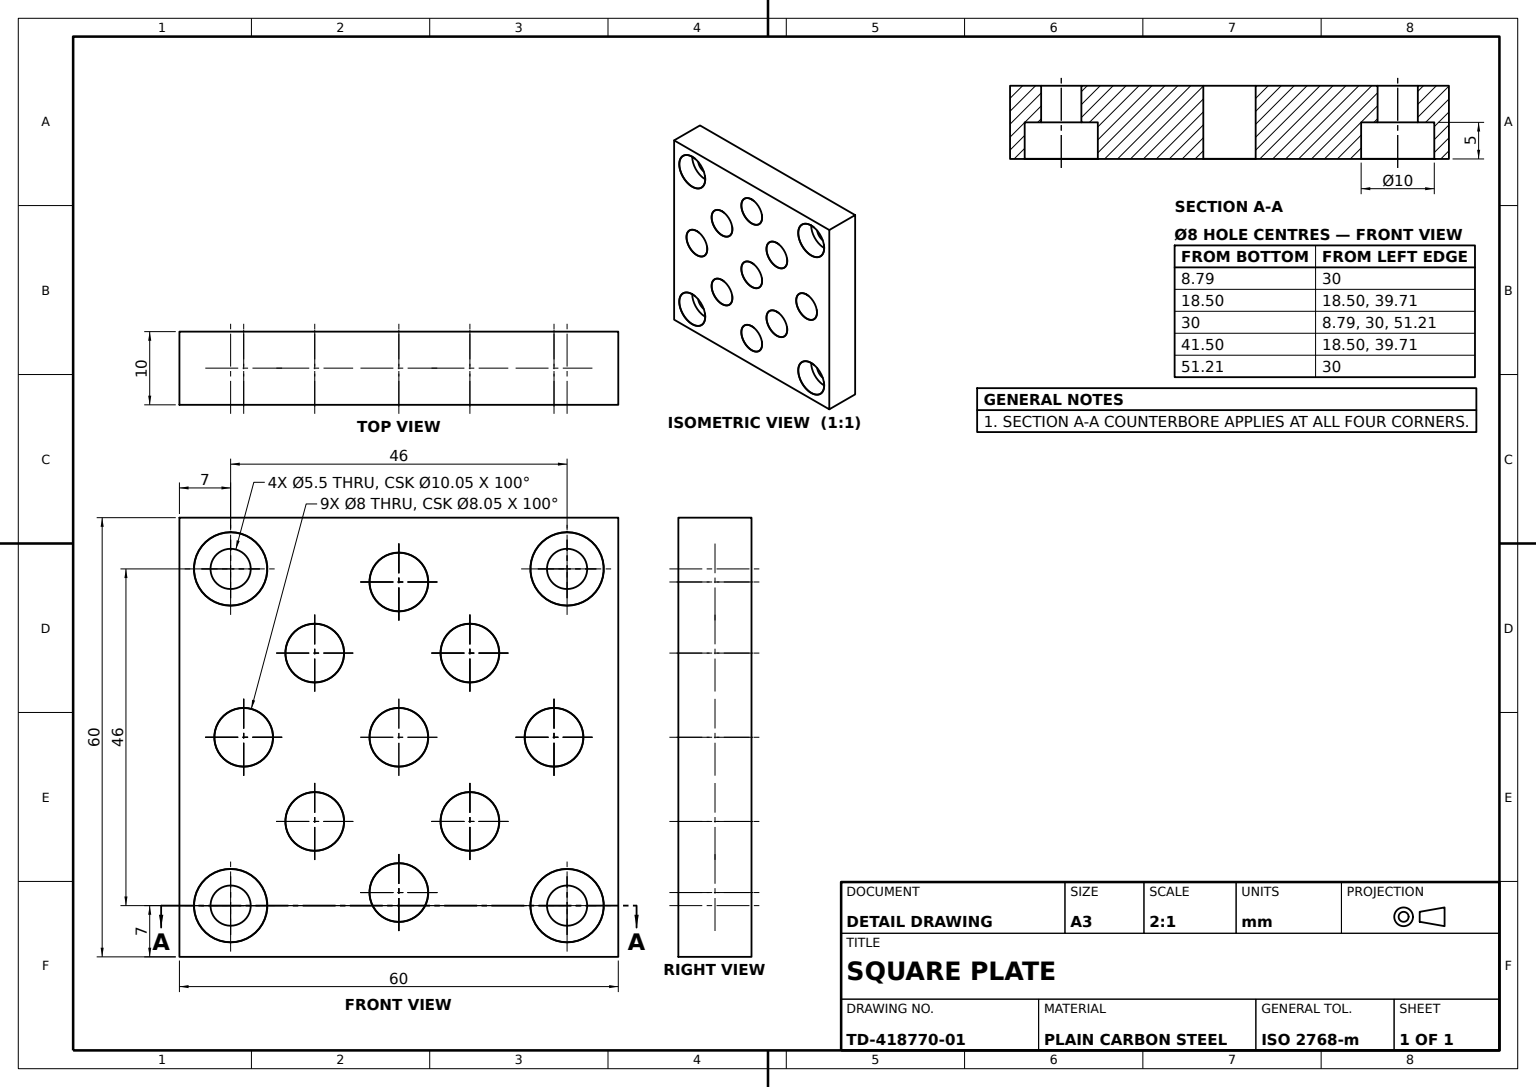
SolidWorks part; units mm, degrees
material "Plain Carbon Steel"
ref_plane "Front Plane" through (0, 0, 0) normal (0, 0, 1) x (1, 0, 0)
ref_plane "Top Plane" through (0, 0, 0) normal (0, 1, 0) x (1, 0, 0)
ref_plane "Right Plane" through (0, 0, 0) normal (1, 0, 0) x (0, 0, -1)
sketch "Base Plate Profile" plane through (0, 0, 0) normal (0, 1, 0) x (1, 0, 0)
  line L1 (30, 30) -> (-30, 30)
  line L2 (30, 30) -> (30, -30)
  line L3 (30, -30) -> (-30, -30)
  line L4 (-30, 30) -> (-30, -30)
  line L5 (30, 30) -> (-30, -30) construction
  line L6 (30, -30) -> (-30, 30) construction
  point P0 (0, 0)
  dimension "D1" = 60
  dimension "D2" = 60
extrude "Base Plate 60x60x10" add sketch "Base Plate Profile" along normal blind 10
sketch "Hole Layout Sketch" plane through (0, 10, 0) normal (0, 1, 0) x (1, 0, 0)
  line L0 (-41.5877, 62.8009) -> (39.8009, -18.5877) construction
  line L1 (30, 30) -> (-30, 30) construction
  line L2 (-38.6074, 0) -> (35.7686, 0) construction
  line L3 (-38.6074, -23) -> (38.6074, -23) construction
  line L4 (-38.6074, 23) -> (38.6074, 23) construction
  line L5 (0, 34.5621) -> (0, -37.117) construction
  line L6 (-30, 30) -> (40.6144, -40.6144) construction
  line L7 (-62.8009, 41.5877) -> (18.5877, -39.8009) construction
  line L9 (-30, 30) -> (-30, -30) construction
  point P16 (23, -23)
  point P18 (23, 23)
  point P19 (-23, 23)
  point P23 (-23, -23)
  dimension "D1" = 30
  dimension "D2" = 46
  dimension "D3" = 7
  dimension "D4" = 45
  dimension "D5" = 46
  dimension "D6" = 7
hole_wizard "Corner Counterbores M5 SHCS" positions "3DSketch1" profile "Sketch3" counterbore size "M5" standard "ANSI Metric"
sketch3d "3DSketch1"
  point P0 (-23, 10, -23)
  point P3 (23, 10, -23)
  point P6 (23, 10, 23)
  point P9 (-23, 10, 23)
sketch "Sketch3" plane through (-23, 10, -23) normal (1, 0, 0) x (0, 0, 1)
  line L0 (0, 0) -> (0, 38)
  line L1 (0, 38) -> (2.75, 36.3476)
  line L2 (2.75, 36.3476) -> (2.75, 5)
  line L3 (2.75, 5) -> (5, 5)
  line L5 (5, 5) -> (5, 0.021)
  line L6 (5, 0.021) -> (5.025, 0)
  line L7 (5.025, 0) -> (0, 0)
  line L8 (-5, 0.021) -> (-5.025, 0) construction
  line L10 (0, 38) -> (-2.75, 36.3476) construction
  line L11 (0, -6.35) -> (0, 107.95) construction
  dimension "Hole Dia." = 5.5
  dimension "Hole Depth" = 38
  dimension "C'Bore Dia." = 10
  dimension "C'Bore Depth" = 5
  dimension "Near C'Sink Dia." = 10.05
  dimension "Near C'Sink Angle" = 100
  dimension "Drill Angle" = 118
sketch "Dowel Hole Grid Sketch" plane through (0, 10, 0) normal (0, 1, 0) x (1, 0, 0)
  line L0 (-38.6074, 0) -> (35.7686, 0) construction
  line L1 (-62.8009, 41.5877) -> (18.5877, -39.8009) construction
  line L2 (-41.5877, 62.8009) -> (39.8009, -18.5877) construction
  line L3 (-30, 30) -> (40.6144, -40.6144) construction
  line L4 (-38.6074, 23) -> (38.6074, 23) construction
  line L5 (0, 34.5621) -> (0, -37.117) construction
  line L6 (-45.2132, 0) -> (38.6001, 0) construction
  circle A0 centre (-21.2132, 0) radius 4
  circle A1 centre (0, 0) radius 4
  circle A2 centre (21.2132, 0) radius 4
  circle A3 centre (-11.5, 11.5) radius 4
  circle A4 centre (9.7132, 11.5) radius 4
  circle A5 centre (0, 21.2132) radius 4
  circle A6 centre (-11.5, -11.5) radius 4
  circle A7 centre (9.7132, -11.5) radius 4
  circle A8 centre (0, -21.2132) radius 4
  point P0 (-21.2132, 0)
  point P6 (0, 0)
  point P9 (21.2132, 0)
  point P13 (-11.5, 11.5)
  point P18 (-11.5, 11.5)
  point P20 (9.7132, 11.5)
  point P22 (0, 21.2132)
  point P23 (0, 21.2132)
  point P29 (-11.5, -11.5)
  point P31 (9.7132, -11.5)
  point P33 (0, -21.2132)
  dimension "D1" = 8
  dimension "D2" = 11.5
hole_wizard "Dowel Hole Grid Ø8" positions "Dowel Hole Grid Sketch" profile "Sketch5" hole size "Ø8.0" standard "ANSI Metric"
sketch "Sketch5" plane through (-21.2132, 10, 0) normal (1, 0, 0) x (0, 0, 1)
  line L0 (0, 0) -> (0, 38)
  line L1 (0, 38) -> (4, 35.5966)
  line L2 (4, 35.5966) -> (4, 0.021)
  line L3 (4, 0.021) -> (4.025, 0)
  line L5 (4.025, 0) -> (0, 0)
  line L6 (-4, 0.021) -> (-4.025, 0) construction
  line L10 (0, 38) -> (-4, 35.5966) construction
  line L11 (0, -6.35) -> (0, 107.95) construction
  dimension "Hole Dia." = 8
  dimension "Hole Depth" = 38
  dimension "Near C'Sink Dia." = 8.05
  dimension "Near C'Sink Angle" = 100
  dimension "Drill Angle" = 118
